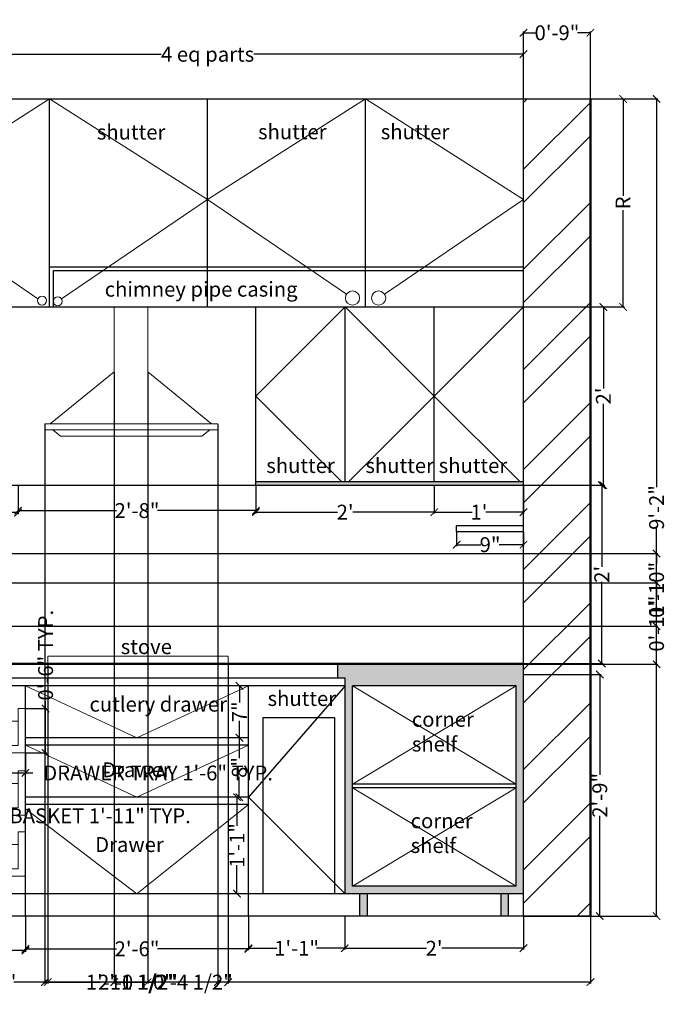
# Model space of a CAD drawing. Units: inches. Extents: x 3107 to 3291, y 1339 to 1621.
# Tile 3 of 3: x 3204 to 3291, y 1489 to 1621. Entities that reach past the tile are written whole.
import ezdxf

# ---------------------------------------------------------------- set-up
doc = ezdxf.new("R2010")
doc.units = ezdxf.units.IN
for name, color, linetype, lineweight in [('A-ANNO-DIMS', 2, 'Continuous', 18), ('A-ANNO-TEXT', 7, 'Continuous', 18), ('A-ELEV', 7, 'Continuous', 25), ('A-ELEV-OPEN', 165, 'Continuous', 13), ('A-ELEV-PATT', 8, 'Continuous', 13), ('A-EQPM', 3, 'Continuous', 18), ('A-FURN', 5, 'Continuous', 18), ('A-WALL', 7, 'Continuous', 50), ('A-WALL-PATT', 8, 'Continuous', 13)]:
    doc.layers.add(name, color=color, linetype=linetype, lineweight=lineweight)
doc.styles.get("Standard").update_dxf_attribs({"font": 'arial.ttf', "height": 2})
doc.dimstyles.get("Standard").update_dxf_attribs({"dimtxt": 2, "dimasz": 1, "dimexe": 0.18, "dimexo": 0.0625, "dimgap": 0.09, "dimtad": 0, "dimdec": 0, "dimzin": 0, "dimdsep": 46, "dimlunit": 3, "dimtxsty": 'Standard', "dimblk": 'ARCHTICK', "dimcen": 0.09, "dimadec": 0, "dimazin": 0, "dimtfac": 1, "dimtdec": 0, "dimtofl": 0, "dimtmove": 0, "dimatfit": 3, "dimfxl": 1, "dimtolj": 1, "dimtzin": 0, "dimarcsym": 0})

# ---------------------------------------------------------------- blocks, each defined once
blk = doc.blocks.new('_ArchTick')
at = {"color": 0, "linetype": 'ByBlock', "const_width": 0.15}
blk.add_lwpolyline([(-0.5, -0.5), (0.5, 0.5)], dxfattribs=at)
blk = doc.blocks.new('*D20')
at = {"layer": 'A-ANNO-DIMS', "color": 0, "lineweight": -2, "transparency": 16777216}
for p, q in [((3259.52, 1558.6), (3259.52, 1554.85)), ((3271.52, 1558.6), (3271.52, 1554.85)), ((3259.52, 1555.03), (3264.6, 1555.03)), ((3271.52, 1555.03), (3266.43, 1555.03))]:
    blk.add_line(p, q, dxfattribs=at)
at = {"layer": 'Defpoints', "color": 0, "transparency": 16777216}
for p in [(3259.52, 1558.66), (3271.52, 1558.66), (3259.52, 1555.03)]:
    blk.add_point(p, dxfattribs=at)
at = {"layer": 'A-ANNO-DIMS', "color": 0, "lineweight": -2, "transparency": 16777216, "rotation": 180}
blk.add_blockref('_ArchTick', (3259.52, 1555.03), dxfattribs=at)
at = {"layer": 'A-ANNO-DIMS', "color": 0, "lineweight": -2, "transparency": 16777216}
blk.add_blockref('_ArchTick', (3271.52, 1555.03), dxfattribs=at)
at = {"layer": 'A-ANNO-DIMS', "color": 0, "transparency": 16777216, "insert": (3265.52, 1555.03), "char_height": 2, "attachment_point": 5}
blk.add_mtext("\\A1;1'", dxfattribs=at)
blk = doc.blocks.new('*D21')
at = {"layer": 'A-ANNO-DIMS', "color": 0, "lineweight": -2, "transparency": 16777216}
for p, q in [((3235.52, 1558.6), (3235.52, 1554.85)), ((3259.52, 1558.6), (3259.52, 1554.85)), ((3235.52, 1555.03), (3246.49, 1555.03)), ((3259.52, 1555.03), (3248.54, 1555.03))]:
    blk.add_line(p, q, dxfattribs=at)
at = {"layer": 'Defpoints', "color": 0, "transparency": 16777216}
for p in [(3235.52, 1558.66), (3259.52, 1558.66), (3235.52, 1555.03)]:
    blk.add_point(p, dxfattribs=at)
at = {"layer": 'A-ANNO-DIMS', "color": 0, "lineweight": -2, "transparency": 16777216, "rotation": 180}
blk.add_blockref('_ArchTick', (3235.52, 1555.03), dxfattribs=at)
at = {"layer": 'A-ANNO-DIMS', "color": 0, "lineweight": -2, "transparency": 16777216}
blk.add_blockref('_ArchTick', (3259.52, 1555.03), dxfattribs=at)
at = {"layer": 'A-ANNO-DIMS', "color": 0, "transparency": 16777216, "insert": (3247.52, 1555.03), "char_height": 2, "attachment_point": 5}
blk.add_mtext("\\A1;2'", dxfattribs=at)
blk = doc.blocks.new('*D22')
at = {"layer": 'A-ANNO-DIMS', "color": 0, "lineweight": -2, "transparency": 16777216}
for p, q in [((3203.52, 1558.6), (3203.52, 1555.06)), ((3235.52, 1558.6), (3235.52, 1555.06)), ((3203.52, 1555.24), (3216.75, 1555.24)), ((3235.52, 1555.24), (3222.28, 1555.24))]:
    blk.add_line(p, q, dxfattribs=at)
at = {"layer": 'Defpoints', "color": 0, "transparency": 16777216}
for p in [(3203.52, 1558.66), (3235.52, 1558.66), (3203.52, 1555.24)]:
    blk.add_point(p, dxfattribs=at)
at = {"layer": 'A-ANNO-DIMS', "color": 0, "lineweight": -2, "transparency": 16777216, "rotation": 180}
blk.add_blockref('_ArchTick', (3203.52, 1555.24), dxfattribs=at)
at = {"layer": 'A-ANNO-DIMS', "color": 0, "lineweight": -2, "transparency": 16777216}
blk.add_blockref('_ArchTick', (3235.52, 1555.24), dxfattribs=at)
at = {"layer": 'A-ANNO-DIMS', "color": 0, "transparency": 16777216, "insert": (3219.52, 1555.24), "char_height": 2, "attachment_point": 5}
blk.add_mtext('\\A1;2\'-8"', dxfattribs=at)
blk = doc.blocks.new('*D23')
at = {"layer": 'A-ANNO-DIMS', "color": 0, "lineweight": -2, "transparency": 16777216}
for p, q in [((3186.52, 1558.6), (3186.52, 1554.78)), ((3203.52, 1558.6), (3203.52, 1554.78)), ((3186.52, 1554.96), (3192.36, 1554.96)), ((3203.52, 1554.96), (3197.67, 1554.96))]:
    blk.add_line(p, q, dxfattribs=at)
at = {"layer": 'Defpoints', "color": 0, "transparency": 16777216}
for p in [(3186.52, 1558.66), (3203.52, 1558.66), (3186.52, 1554.96)]:
    blk.add_point(p, dxfattribs=at)
at = {"layer": 'A-ANNO-DIMS', "color": 0, "lineweight": -2, "transparency": 16777216, "rotation": 180}
blk.add_blockref('_ArchTick', (3186.52, 1554.96), dxfattribs=at)
at = {"layer": 'A-ANNO-DIMS', "color": 0, "lineweight": -2, "transparency": 16777216}
blk.add_blockref('_ArchTick', (3203.52, 1554.96), dxfattribs=at)
at = {"layer": 'A-ANNO-DIMS', "color": 0, "transparency": 16777216, "insert": (3195.02, 1554.96), "char_height": 2, "attachment_point": 5}
blk.add_mtext('\\A1;1\'-5"', dxfattribs=at)
blk = doc.blocks.new('*D24')
at = {"layer": 'A-ANNO-DIMS', "color": 0, "lineweight": -2, "transparency": 16777216}
for p, q in [((3247.47, 1500.6), (3247.47, 1496.14)), ((3271.52, 1500.6), (3271.52, 1496.14)), ((3247.47, 1496.32), (3258.47, 1496.32)), ((3271.52, 1496.32), (3260.52, 1496.32))]:
    blk.add_line(p, q, dxfattribs=at)
at = {"layer": 'Defpoints', "color": 0, "transparency": 16777216}
for p in [(3247.47, 1500.66), (3271.52, 1500.66), (3247.47, 1496.32)]:
    blk.add_point(p, dxfattribs=at)
at = {"layer": 'A-ANNO-DIMS', "color": 0, "lineweight": -2, "transparency": 16777216, "rotation": 180}
blk.add_blockref('_ArchTick', (3247.47, 1496.32), dxfattribs=at)
at = {"layer": 'A-ANNO-DIMS', "color": 0, "lineweight": -2, "transparency": 16777216}
blk.add_blockref('_ArchTick', (3271.52, 1496.32), dxfattribs=at)
at = {"layer": 'A-ANNO-DIMS', "color": 0, "transparency": 16777216, "insert": (3259.49, 1496.32), "char_height": 2, "attachment_point": 5}
blk.add_mtext("\\A1;2'", dxfattribs=at)
blk = doc.blocks.new('*D25')
at = {"layer": 'A-ANNO-DIMS', "color": 0, "lineweight": -2, "transparency": 16777216}
for p, q in [((3234.52, 1500.6), (3234.52, 1496.14)), ((3247.47, 1500.6), (3247.47, 1496.14)), ((3234.52, 1496.32), (3238.34, 1496.32)), ((3247.47, 1496.32), (3243.65, 1496.32))]:
    blk.add_line(p, q, dxfattribs=at)
at = {"layer": 'Defpoints', "color": 0, "transparency": 16777216}
for p in [(3234.52, 1500.66), (3247.47, 1500.66), (3234.52, 1496.32)]:
    blk.add_point(p, dxfattribs=at)
at = {"layer": 'A-ANNO-DIMS', "color": 0, "lineweight": -2, "transparency": 16777216, "rotation": 180}
blk.add_blockref('_ArchTick', (3234.52, 1496.32), dxfattribs=at)
at = {"layer": 'A-ANNO-DIMS', "color": 0, "lineweight": -2, "transparency": 16777216}
blk.add_blockref('_ArchTick', (3247.47, 1496.32), dxfattribs=at)
at = {"layer": 'A-ANNO-DIMS', "color": 0, "transparency": 16777216, "insert": (3240.99, 1496.32), "char_height": 2, "attachment_point": 5}
blk.add_mtext('\\A1;1\'-1"', dxfattribs=at)
blk = doc.blocks.new('*D26')
at = {"layer": 'A-ANNO-DIMS', "color": 0, "lineweight": -2, "transparency": 16777216}
for p, q in [((3204.52, 1500.6), (3204.52, 1496.07)), ((3234.52, 1500.6), (3234.52, 1496.07)), ((3204.52, 1496.25), (3216.75, 1496.25)), ((3234.52, 1496.25), (3222.28, 1496.25))]:
    blk.add_line(p, q, dxfattribs=at)
at = {"layer": 'Defpoints', "color": 0, "transparency": 16777216}
for p in [(3204.52, 1500.66), (3234.52, 1500.66), (3204.52, 1496.25)]:
    blk.add_point(p, dxfattribs=at)
at = {"layer": 'A-ANNO-DIMS', "color": 0, "lineweight": -2, "transparency": 16777216, "rotation": 180}
blk.add_blockref('_ArchTick', (3204.52, 1496.25), dxfattribs=at)
at = {"layer": 'A-ANNO-DIMS', "color": 0, "lineweight": -2, "transparency": 16777216}
blk.add_blockref('_ArchTick', (3234.52, 1496.25), dxfattribs=at)
at = {"layer": 'A-ANNO-DIMS', "color": 0, "transparency": 16777216, "insert": (3219.52, 1496.25), "char_height": 2, "attachment_point": 5}
blk.add_mtext('\\A1;2\'-6"', dxfattribs=at)
blk = doc.blocks.new('*D27')
at = {"layer": 'A-ANNO-DIMS', "color": 0, "lineweight": -2, "transparency": 16777216}
for p, q in [((3186.52, 1500.6), (3186.52, 1495.83)), ((3204.52, 1500.6), (3204.52, 1495.83)), ((3186.52, 1496.01), (3192.86, 1496.01)), ((3204.52, 1496.01), (3198.17, 1496.01))]:
    blk.add_line(p, q, dxfattribs=at)
at = {"layer": 'Defpoints', "color": 0, "transparency": 16777216}
for p in [(3186.52, 1500.66), (3204.52, 1500.66), (3186.52, 1496.01)]:
    blk.add_point(p, dxfattribs=at)
at = {"layer": 'A-ANNO-DIMS', "color": 0, "lineweight": -2, "transparency": 16777216, "rotation": 180}
blk.add_blockref('_ArchTick', (3186.52, 1496.01), dxfattribs=at)
at = {"layer": 'A-ANNO-DIMS', "color": 0, "lineweight": -2, "transparency": 16777216}
blk.add_blockref('_ArchTick', (3204.52, 1496.01), dxfattribs=at)
at = {"layer": 'A-ANNO-DIMS', "color": 0, "transparency": 16777216, "insert": (3195.52, 1496.01), "char_height": 2, "attachment_point": 5}
blk.add_mtext('\\A1;1\'-6"', dxfattribs=at)
blk = doc.blocks.new('*D30')
at = {"layer": 'A-ANNO-DIMS', "color": 0, "lineweight": -2, "transparency": 16777216}
for p, q in [((3271.58, 1533.17), (3281.96, 1533.17)), ((3281.78, 1533.17), (3281.78, 1519.68)), ((3281.78, 1500.66), (3281.78, 1514.15)), ((3271.58, 1500.66), (3281.96, 1500.66))]:
    blk.add_line(p, q, dxfattribs=at)
at = {"layer": 'Defpoints', "color": 0, "transparency": 16777216}
for p in [(3271.52, 1533.17), (3281.78, 1533.17), (3271.52, 1500.66)]:
    blk.add_point(p, dxfattribs=at)
at = {"layer": 'A-ANNO-DIMS', "color": 0, "lineweight": -2, "transparency": 16777216}
for p, rotation in [((3281.78, 1533.17), 90), ((3281.78, 1500.66), 270)]:
    blk.add_blockref('_ArchTick', p, dxfattribs=dict(at, rotation=rotation))
at = {"layer": 'A-ANNO-DIMS', "color": 0, "transparency": 16777216, "insert": (3281.78, 1516.91), "char_height": 2, "attachment_point": 5, "rotation": 90}
blk.add_mtext('\\A1;2\'-9"', dxfattribs=at)
blk = doc.blocks.new('*D31')
at = {"layer": 'A-ANNO-DIMS', "color": 0, "lineweight": -2, "transparency": 16777216}
for p, q in [((3271.58, 1558.66), (3282.23, 1558.66)), ((3282.05, 1558.66), (3282.05, 1547.69)), ((3282.05, 1534.66), (3282.05, 1545.63)), ((3271.58, 1534.66), (3282.23, 1534.66))]:
    blk.add_line(p, q, dxfattribs=at)
at = {"layer": 'Defpoints', "color": 0, "transparency": 16777216}
for p in [(3271.52, 1558.66), (3282.05, 1558.66), (3271.52, 1534.66)]:
    blk.add_point(p, dxfattribs=at)
at = {"layer": 'A-ANNO-DIMS', "color": 0, "lineweight": -2, "transparency": 16777216}
for p, rotation in [((3282.05, 1558.66), 90), ((3282.05, 1534.66), 270)]:
    blk.add_blockref('_ArchTick', p, dxfattribs=dict(at, rotation=rotation))
at = {"layer": 'A-ANNO-DIMS', "color": 0, "transparency": 16777216, "insert": (3282.05, 1546.66), "char_height": 2, "attachment_point": 5, "rotation": 90}
blk.add_mtext("\\A1;2'", dxfattribs=at)
blk = doc.blocks.new('*D32')
at = {"layer": 'A-ANNO-DIMS', "color": 0, "lineweight": -2, "transparency": 16777216}
for p, q in [((3271.58, 1582.66), (3282.44, 1582.66)), ((3282.26, 1582.66), (3282.26, 1571.69)), ((3282.26, 1558.66), (3282.26, 1569.63)), ((3271.58, 1558.66), (3282.44, 1558.66))]:
    blk.add_line(p, q, dxfattribs=at)
at = {"layer": 'Defpoints', "color": 0, "transparency": 16777216}
for p in [(3271.52, 1582.66), (3282.26, 1582.66), (3271.52, 1558.66)]:
    blk.add_point(p, dxfattribs=at)
at = {"layer": 'A-ANNO-DIMS', "color": 0, "lineweight": -2, "transparency": 16777216}
for p, rotation in [((3282.26, 1582.66), 90), ((3282.26, 1558.66), 270)]:
    blk.add_blockref('_ArchTick', p, dxfattribs=dict(at, rotation=rotation))
at = {"layer": 'A-ANNO-DIMS', "color": 0, "transparency": 16777216, "insert": (3282.26, 1570.66), "char_height": 2, "attachment_point": 5, "rotation": 90}
blk.add_mtext("\\A1;2'", dxfattribs=at)
blk = doc.blocks.new('*D33')
at = {"layer": 'A-ANNO-DIMS', "color": 0, "lineweight": -2, "transparency": 16777216}
for p, q in [((3271.58, 1610.66), (3285.09, 1610.66)), ((3284.91, 1610.66), (3284.91, 1597.63)), ((3284.91, 1582.66), (3284.91, 1595.69)), ((3271.58, 1582.66), (3285.09, 1582.66))]:
    blk.add_line(p, q, dxfattribs=at)
at = {"layer": 'Defpoints', "color": 0, "transparency": 16777216}
for p in [(3271.52, 1610.66), (3284.91, 1610.66), (3271.52, 1582.66)]:
    blk.add_point(p, dxfattribs=at)
at = {"layer": 'A-ANNO-DIMS', "color": 0, "lineweight": -2, "transparency": 16777216}
for p, rotation in [((3284.91, 1610.66), 90), ((3284.91, 1582.66), 270)]:
    blk.add_blockref('_ArchTick', p, dxfattribs=dict(at, rotation=rotation))
at = {"layer": 'A-ANNO-DIMS', "color": 0, "transparency": 16777216, "insert": (3284.91, 1596.66), "char_height": 2, "attachment_point": 5, "rotation": 90}
blk.add_mtext('\\A1;R ', dxfattribs=at)
blk = doc.blocks.new('*D34')
at = {"layer": 'A-ANNO-DIMS', "color": 0, "lineweight": -2, "transparency": 16777216}
for p, q in [((3186.52, 1610.72), (3186.52, 1616.85)), ((3186.52, 1616.67), (3222.79, 1616.67)), ((3271.52, 1616.67), (3235.25, 1616.67)), ((3271.52, 1610.72), (3271.52, 1616.85))]:
    blk.add_line(p, q, dxfattribs=at)
at = {"layer": 'Defpoints', "color": 0, "transparency": 16777216}
for p in [(3186.52, 1616.67), (3186.52, 1610.66), (3271.52, 1610.66)]:
    blk.add_point(p, dxfattribs=at)
at = {"layer": 'A-ANNO-DIMS', "color": 0, "lineweight": -2, "transparency": 16777216, "rotation": 180}
blk.add_blockref('_ArchTick', (3186.52, 1616.67), dxfattribs=at)
at = {"layer": 'A-ANNO-DIMS', "color": 0, "lineweight": -2, "transparency": 16777216}
blk.add_blockref('_ArchTick', (3271.52, 1616.67), dxfattribs=at)
at = {"layer": 'A-ANNO-DIMS', "color": 0, "transparency": 16777216, "insert": (3229.02, 1616.67), "char_height": 2, "attachment_point": 5}
blk.add_mtext('\\A1;4 eq parts', dxfattribs=at)
blk = doc.blocks.new('*D39')
at = {"layer": 'A-ANNO-DIMS', "color": 0, "lineweight": -2, "transparency": 16777216}
for p, q in [((3262.52, 1552.37), (3262.52, 1550.47)), ((3271.52, 1552.37), (3271.52, 1550.47)), ((3262.52, 1550.65), (3265.78, 1550.65)), ((3271.52, 1550.65), (3268.26, 1550.65))]:
    blk.add_line(p, q, dxfattribs=at)
at = {"layer": 'Defpoints', "color": 0, "transparency": 16777216}
for p in [(3262.52, 1552.43), (3271.52, 1552.43), (3262.52, 1550.65)]:
    blk.add_point(p, dxfattribs=at)
at = {"layer": 'A-ANNO-DIMS', "color": 0, "lineweight": -2, "transparency": 16777216, "rotation": 180}
blk.add_blockref('_ArchTick', (3262.52, 1550.65), dxfattribs=at)
at = {"layer": 'A-ANNO-DIMS', "color": 0, "lineweight": -2, "transparency": 16777216}
blk.add_blockref('_ArchTick', (3271.52, 1550.65), dxfattribs=at)
at = {"layer": 'A-ANNO-DIMS', "color": 0, "transparency": 16777216, "insert": (3267.02, 1550.65), "char_height": 2, "attachment_point": 5}
blk.add_mtext('\\A1;9"', dxfattribs=at)
blk = doc.blocks.new('*D45')
at = {"layer": 'A-ANNO-DIMS', "color": 0, "lineweight": -2, "transparency": 16777216}
for p, q in [((3234.46, 1531.66), (3233.13, 1531.66)), ((3233.31, 1531.66), (3233.31, 1529.39)), ((3233.31, 1524.66), (3233.31, 1526.93)), ((3234.46, 1524.66), (3233.13, 1524.66))]:
    blk.add_line(p, q, dxfattribs=at)
at = {"layer": 'Defpoints', "color": 0, "transparency": 16777216}
for p in [(3233.31, 1531.66), (3234.52, 1531.66), (3234.52, 1524.66)]:
    blk.add_point(p, dxfattribs=at)
at = {"layer": 'A-ANNO-DIMS', "color": 0, "lineweight": -2, "transparency": 16777216}
for p, rotation in [((3233.31, 1531.66), 90), ((3233.31, 1524.66), 270)]:
    blk.add_blockref('_ArchTick', p, dxfattribs=dict(at, rotation=rotation))
at = {"layer": 'A-ANNO-DIMS', "color": 0, "transparency": 16777216, "insert": (3233.31, 1528.16), "char_height": 2, "attachment_point": 5, "rotation": 90}
blk.add_mtext('\\A1;7"', dxfattribs=at)
blk = doc.blocks.new('*D46')
at = {"layer": 'A-ANNO-DIMS', "color": 0, "lineweight": -2, "transparency": 16777216}
for p, q in [((3234.46, 1524.66), (3233.1, 1524.66)), ((3233.28, 1524.66), (3233.28, 1521.9)), ((3233.28, 1516.66), (3233.28, 1519.42)), ((3234.46, 1516.66), (3233.1, 1516.66))]:
    blk.add_line(p, q, dxfattribs=at)
at = {"layer": 'Defpoints', "color": 0, "transparency": 16777216}
for p in [(3234.52, 1524.66), (3233.28, 1516.66), (3234.52, 1516.66)]:
    blk.add_point(p, dxfattribs=at)
at = {"layer": 'A-ANNO-DIMS', "color": 0, "lineweight": -2, "transparency": 16777216}
for p, rotation in [((3233.28, 1524.66), 90), ((3233.28, 1516.66), 270)]:
    blk.add_blockref('_ArchTick', p, dxfattribs=dict(at, rotation=rotation))
at = {"layer": 'A-ANNO-DIMS', "color": 0, "transparency": 16777216, "insert": (3233.28, 1520.66), "char_height": 2, "attachment_point": 5, "rotation": 90}
blk.add_mtext('\\A1;8"', dxfattribs=at)
blk = doc.blocks.new('*D47')
at = {"layer": 'A-ANNO-DIMS', "color": 0, "lineweight": -2, "transparency": 16777216}
for p, q in [((3234.46, 1516.66), (3232.79, 1516.66)), ((3232.97, 1516.66), (3232.97, 1512.81)), ((3232.97, 1503.66), (3232.97, 1507.5)), ((3234.46, 1503.66), (3232.79, 1503.66))]:
    blk.add_line(p, q, dxfattribs=at)
at = {"layer": 'Defpoints', "color": 0, "transparency": 16777216}
for p in [(3234.52, 1516.66), (3232.97, 1503.66), (3234.52, 1503.66)]:
    blk.add_point(p, dxfattribs=at)
at = {"layer": 'A-ANNO-DIMS', "color": 0, "lineweight": -2, "transparency": 16777216}
for p, rotation in [((3232.97, 1516.66), 90), ((3232.97, 1503.66), 270)]:
    blk.add_blockref('_ArchTick', p, dxfattribs=dict(at, rotation=rotation))
at = {"layer": 'A-ANNO-DIMS', "color": 0, "transparency": 16777216, "insert": (3232.97, 1510.16), "char_height": 2, "attachment_point": 5, "rotation": 90}
blk.add_mtext('\\A1;1\'-1"', dxfattribs=at)
blk = doc.blocks.new('DRAWER-TRAY')
for p, q in [((3186.52, 1528.59), (3187.52, 1528.59)), ((3186.52, 1522.62), (3186.52, 1528.59)), ((3187.52, 1523.62), (3187.52, 1528.59)), ((3203.52, 1528.59), (3203.52, 1523.62)), ((3203.52, 1528.59), (3204.52, 1528.59)), ((3204.52, 1528.59), (3204.52, 1522.62)), ((3187.52, 1526.9), (3203.52, 1526.9)), ((3203.52, 1523.62), (3187.52, 1523.62)), ((3204.52, 1522.62), (3186.52, 1522.62))]:
    blk.add_line(p, q)
blk = doc.blocks.new('*D50')
at = {"layer": 'A-ANNO-DIMS', "color": 0, "lineweight": -2, "transparency": 16777216}
for p, q in [((3186.52, 1522.56), (3186.52, 1519.74)), ((3204.52, 1522.56), (3204.52, 1519.74)), ((3186.52, 1519.92), (3204.52, 1519.92)), ((3204.52, 1519.92), (3205.52, 1519.92))]:
    blk.add_line(p, q, dxfattribs=at)
at = {"layer": 'Defpoints', "color": 0, "transparency": 16777216}
for p in [(3186.52, 1522.62), (3204.52, 1522.62), (3204.52, 1519.92)]:
    blk.add_point(p, dxfattribs=at)
at = {"layer": 'A-ANNO-DIMS', "color": 0, "lineweight": -2, "transparency": 16777216, "rotation": 180}
blk.add_blockref('_ArchTick', (3186.52, 1519.92), dxfattribs=at)
at = {"layer": 'A-ANNO-DIMS', "color": 0, "lineweight": -2, "transparency": 16777216}
blk.add_blockref('_ArchTick', (3204.52, 1519.92), dxfattribs=at)
at = {"layer": 'A-ANNO-DIMS', "color": 0, "transparency": 16777216, "insert": (3222.36, 1519.92), "char_height": 2, "attachment_point": 5}
blk.add_mtext('\\A1;DRAWER TRAY 1\'-6" TYP.', dxfattribs=at)
blk = doc.blocks.new('*D51')
at = {"layer": 'A-ANNO-DIMS', "color": 0, "lineweight": -2, "transparency": 16777216}
for p, q in [((3204.58, 1528.59), (3207.4, 1528.59)), ((3207.22, 1528.59), (3207.22, 1529.59)), ((3207.22, 1522.62), (3207.22, 1528.59)), ((3204.58, 1522.62), (3207.4, 1522.62))]:
    blk.add_line(p, q, dxfattribs=at)
at = {"layer": 'Defpoints', "color": 0, "transparency": 16777216}
for p in [(3204.52, 1528.59), (3207.22, 1528.59), (3204.52, 1522.62)]:
    blk.add_point(p, dxfattribs=at)
at = {"layer": 'A-ANNO-DIMS', "color": 0, "lineweight": -2, "transparency": 16777216}
for p, rotation in [((3207.22, 1528.59), 90), ((3207.22, 1522.62), 270)]:
    blk.add_blockref('_ArchTick', p, dxfattribs=dict(at, rotation=rotation))
at = {"layer": 'A-ANNO-DIMS', "color": 0, "transparency": 16777216, "insert": (3207.22, 1535.77), "char_height": 2, "attachment_point": 5, "rotation": 90}
blk.add_mtext('\\A1;0\'-6" TYP.', dxfattribs=at)
blk = doc.blocks.new('*D52')
at = {"layer": 'A-ANNO-DIMS', "color": 0, "lineweight": -2, "transparency": 16777216}
for p, q in [((3163.52, 1517.53), (3163.52, 1513.97)), ((3186.52, 1517.53), (3186.52, 1513.97)), ((3163.52, 1514.15), (3186.52, 1514.15)), ((3186.52, 1514.15), (3187.52, 1514.15))]:
    blk.add_line(p, q, dxfattribs=at)
at = {"layer": 'Defpoints', "color": 0, "transparency": 16777216}
for p in [(3163.52, 1517.6), (3186.52, 1517.6), (3186.52, 1514.15)]:
    blk.add_point(p, dxfattribs=at)
at = {"layer": 'A-ANNO-DIMS', "color": 0, "lineweight": -2, "transparency": 16777216, "rotation": 180}
blk.add_blockref('_ArchTick', (3163.52, 1514.15), dxfattribs=at)
at = {"layer": 'A-ANNO-DIMS', "color": 0, "lineweight": -2, "transparency": 16777216}
blk.add_blockref('_ArchTick', (3186.52, 1514.15), dxfattribs=at)
at = {"layer": 'A-ANNO-DIMS', "color": 0, "transparency": 16777216, "insert": (3207.63, 1514.15), "char_height": 2, "attachment_point": 5}
blk.add_mtext('\\A1;PULL-OUT BASKET 1\'-11" TYP.', dxfattribs=at)
blk = doc.blocks.new('*D56')
at = {"layer": 'A-ANNO-DIMS', "color": 0, "lineweight": -2, "transparency": 16777216}
for p, q in [((3280.58, 1610.66), (3289.6, 1610.66)), ((3289.42, 1610.66), (3289.42, 1558.41)), ((3289.42, 1500.66), (3289.42, 1552.91)), ((3280.58, 1500.66), (3289.6, 1500.66))]:
    blk.add_line(p, q, dxfattribs=at)
at = {"layer": 'Defpoints', "color": 0, "transparency": 16777216}
for p in [(3280.52, 1610.66), (3289.42, 1610.66), (3280.52, 1500.66)]:
    blk.add_point(p, dxfattribs=at)
at = {"layer": 'A-ANNO-DIMS', "color": 0, "lineweight": -2, "transparency": 16777216}
for p, rotation in [((3289.42, 1610.66), 90), ((3289.42, 1500.66), 270)]:
    blk.add_blockref('_ArchTick', p, dxfattribs=dict(at, rotation=rotation))
at = {"layer": 'A-ANNO-DIMS', "color": 0, "transparency": 16777216, "insert": (3289.42, 1555.66), "char_height": 2, "attachment_point": 5, "rotation": 90}
blk.add_mtext('\\A1;9\'-2"', dxfattribs=at)
blk = doc.blocks.new('*D59')
at = {"layer": 'A-ANNO-DIMS', "color": 0, "lineweight": -2, "transparency": 16777216}
for p, q in [((3271.52, 1610.72), (3271.52, 1619.74)), ((3280.52, 1610.72), (3280.52, 1619.74)), ((3271.52, 1619.56), (3273.27, 1619.56)), ((3280.52, 1619.56), (3278.77, 1619.56))]:
    blk.add_line(p, q, dxfattribs=at)
at = {"layer": 'Defpoints', "color": 0, "transparency": 16777216}
for p in [(3280.52, 1619.56), (3271.52, 1610.66), (3280.52, 1610.66)]:
    blk.add_point(p, dxfattribs=at)
at = {"layer": 'A-ANNO-DIMS', "color": 0, "lineweight": -2, "transparency": 16777216, "rotation": 180}
blk.add_blockref('_ArchTick', (3271.52, 1619.56), dxfattribs=at)
at = {"layer": 'A-ANNO-DIMS', "color": 0, "lineweight": -2, "transparency": 16777216}
blk.add_blockref('_ArchTick', (3280.52, 1619.56), dxfattribs=at)
at = {"layer": 'A-ANNO-DIMS', "color": 0, "transparency": 16777216, "insert": (3276.02, 1619.56), "char_height": 2, "attachment_point": 5}
blk.add_mtext('\\A1;0\'-9"', dxfattribs=at)
blk = doc.blocks.new('*D62')
at = {"layer": 'A-ANNO-DIMS', "color": 0, "lineweight": -2, "transparency": 16777216}
for p, q in [((3140.37, 1549.46), (3289.6, 1549.46)), ((3289.42, 1549.46), (3289.42, 1548.09)), ((3289.42, 1539.66), (3289.42, 1541.04)), ((3140.87, 1539.66), (3289.6, 1539.66))]:
    blk.add_line(p, q, dxfattribs=at)
at = {"layer": 'Defpoints', "color": 0, "transparency": 16777216}
for p in [(3140.3, 1549.46), (3289.42, 1549.46), (3140.8, 1539.66)]:
    blk.add_point(p, dxfattribs=at)
at = {"layer": 'A-ANNO-DIMS', "color": 0, "lineweight": -2, "transparency": 16777216}
for p, rotation in [((3289.42, 1549.46), 90), ((3289.42, 1539.66), 270)]:
    blk.add_blockref('_ArchTick', p, dxfattribs=dict(at, rotation=rotation))
at = {"layer": 'A-ANNO-DIMS', "color": 0, "transparency": 16777216, "insert": (3289.42, 1544.56), "char_height": 2, "attachment_point": 5, "rotation": 90}
blk.add_mtext('\\A1;0\'-10"', dxfattribs=at)
blk = doc.blocks.new('*D63')
at = {"layer": 'A-ANNO-DIMS', "color": 0, "lineweight": -2, "transparency": 16777216}
for p, q in [((3184.88, 1545.5), (3289.6, 1545.5)), ((3289.42, 1545.5), (3289.42, 1543.55)), ((3289.42, 1534.55), (3289.42, 1536.5)), ((3184.88, 1534.55), (3289.6, 1534.55))]:
    blk.add_line(p, q, dxfattribs=at)
at = {"layer": 'Defpoints', "color": 0, "transparency": 16777216}
for p in [(3184.82, 1545.5), (3289.42, 1545.5), (3184.82, 1534.55)]:
    blk.add_point(p, dxfattribs=at)
at = {"layer": 'A-ANNO-DIMS', "color": 0, "lineweight": -2, "transparency": 16777216}
for p, rotation in [((3289.42, 1545.5), 90), ((3289.42, 1534.55), 270)]:
    blk.add_blockref('_ArchTick', p, dxfattribs=dict(at, rotation=rotation))
at = {"layer": 'A-ANNO-DIMS', "color": 0, "transparency": 16777216, "insert": (3289.42, 1540.02), "char_height": 2, "attachment_point": 5, "rotation": 90}
blk.add_mtext('\\A1;0\'-11"', dxfattribs=at)
blk = doc.blocks.new('*D64')
at = {"layer": 'A-ANNO-DIMS', "color": 0, "lineweight": -2, "transparency": 16777216}
for p, q in [((3207.13, 1566.85), (3207.13, 1491.58)), ((3230.39, 1566.85), (3230.39, 1491.58)), ((3207.13, 1491.76), (3213, 1491.76)), ((3230.39, 1491.76), (3224.52, 1491.76))]:
    blk.add_line(p, q, dxfattribs=at)
at = {"layer": 'Defpoints', "color": 0, "transparency": 16777216}
for p in [(3207.13, 1566.91), (3230.39, 1566.91), (3230.39, 1491.76)]:
    blk.add_point(p, dxfattribs=at)
at = {"layer": 'A-ANNO-DIMS', "color": 0, "lineweight": -2, "transparency": 16777216, "rotation": 180}
blk.add_blockref('_ArchTick', (3207.13, 1491.76), dxfattribs=at)
at = {"layer": 'A-ANNO-DIMS', "color": 0, "lineweight": -2, "transparency": 16777216}
blk.add_blockref('_ArchTick', (3230.39, 1491.76), dxfattribs=at)
at = {"layer": 'A-ANNO-DIMS', "color": 0, "transparency": 16777216, "insert": (3218.76, 1491.76), "char_height": 2, "attachment_point": 5}
blk.add_mtext('\\A1;1\'-11 1/2"', dxfattribs=at)
blk = doc.blocks.new('*D65')
at = {"layer": 'A-ANNO-DIMS', "color": 0, "lineweight": -2, "transparency": 16777216}
for p, q in [((3216.45, 1573.85), (3216.45, 1491.58)), ((3220.96, 1573.85), (3220.96, 1491.58)), ((3216.45, 1491.76), (3220.96, 1491.76)), ((3220.96, 1491.76), (3221.96, 1491.76))]:
    blk.add_line(p, q, dxfattribs=at)
at = {"layer": 'Defpoints', "color": 0, "transparency": 16777216}
for p in [(3216.45, 1573.91), (3220.96, 1573.91), (3220.96, 1491.76)]:
    blk.add_point(p, dxfattribs=at)
at = {"layer": 'A-ANNO-DIMS', "color": 0, "lineweight": -2, "transparency": 16777216, "rotation": 180}
blk.add_blockref('_ArchTick', (3216.45, 1491.76), dxfattribs=at)
at = {"layer": 'A-ANNO-DIMS', "color": 0, "lineweight": -2, "transparency": 16777216}
blk.add_blockref('_ArchTick', (3220.96, 1491.76), dxfattribs=at)
at = {"layer": 'A-ANNO-DIMS', "color": 0, "transparency": 16777216, "insert": (3227.04, 1491.76), "char_height": 2, "attachment_point": 5}
blk.add_mtext('\\A1;0\'-4 1/2"', dxfattribs=at)
blk = doc.blocks.new('*D66')
at = {"layer": 'A-ANNO-DIMS', "color": 0, "lineweight": -2, "transparency": 16777216}
for p, q in [((3207.51, 1534.6), (3207.51, 1491.58)), ((3231.79, 1534.6), (3231.79, 1491.58)), ((3207.51, 1491.76), (3214.55, 1491.76)), ((3231.79, 1491.76), (3224.75, 1491.76))]:
    blk.add_line(p, q, dxfattribs=at)
at = {"layer": 'Defpoints', "color": 0, "transparency": 16777216}
for p in [(3207.51, 1534.66), (3231.79, 1534.66), (3231.79, 1491.76)]:
    blk.add_point(p, dxfattribs=at)
at = {"layer": 'A-ANNO-DIMS', "color": 0, "lineweight": -2, "transparency": 16777216, "rotation": 180}
blk.add_blockref('_ArchTick', (3207.51, 1491.76), dxfattribs=at)
at = {"layer": 'A-ANNO-DIMS', "color": 0, "lineweight": -2, "transparency": 16777216}
blk.add_blockref('_ArchTick', (3231.79, 1491.76), dxfattribs=at)
at = {"layer": 'A-ANNO-DIMS', "color": 0, "transparency": 16777216, "insert": (3219.65, 1491.76), "char_height": 2, "attachment_point": 5}
blk.add_mtext('\\A1;2\'-0 1/2"', dxfattribs=at)
blk = doc.blocks.new('*D67')
at = {"layer": 'A-ANNO-DIMS', "color": 0, "lineweight": -2, "transparency": 16777216}
for p, q in [((3118.52, 1500.6), (3118.52, 1491.58)), ((3280.52, 1500.6), (3280.52, 1491.58)), ((3118.52, 1491.76), (3196.09, 1491.76)), ((3280.52, 1491.76), (3202.95, 1491.76))]:
    blk.add_line(p, q, dxfattribs=at)
at = {"layer": 'Defpoints', "color": 0, "transparency": 16777216}
for p in [(3118.52, 1500.66), (3280.52, 1500.66), (3280.52, 1491.76)]:
    blk.add_point(p, dxfattribs=at)
at = {"layer": 'A-ANNO-DIMS', "color": 0, "lineweight": -2, "transparency": 16777216, "rotation": 180}
blk.add_blockref('_ArchTick', (3118.52, 1491.76), dxfattribs=at)
at = {"layer": 'A-ANNO-DIMS', "color": 0, "lineweight": -2, "transparency": 16777216}
blk.add_blockref('_ArchTick', (3280.52, 1491.76), dxfattribs=at)
at = {"layer": 'A-ANNO-DIMS', "color": 0, "transparency": 16777216, "insert": (3199.52, 1491.76), "char_height": 2, "attachment_point": 5}
blk.add_mtext('\\A1;13\'-6"', dxfattribs=at)

msp = doc.modelspace()

# ---------------------------------------------------------------- hatches: boundary and pattern name
at = {"layer": 'A-ELEV-PATT'}
h = msp.add_hatch(color=256, dxfattribs=at)
h.dxf.hatch_style = 1
h.paths.add_polyline_path([(3271.52, 1559.16), (3235.52, 1559.16), (3235.52, 1558.66), (3271.52, 1558.66)])
h = msp.add_hatch(color=256, dxfattribs=at)
h.dxf.hatch_style = 1
h.paths.add_polyline_path([(3271.52, 1534.66), (3246.53, 1534.66), (3246.53, 1532.66), (3247.52, 1532.66), (3247.52, 1503.66), (3271.52, 1503.66)])
h.paths.add_polyline_path([(3270.52, 1504.66), (3248.52, 1504.66), (3248.52, 1531.66), (3270.52, 1531.66)], flags=16)
h.paths.add_polyline_path([(3259.52, 1525.03), (3270.52, 1518.41), (3248.52, 1518.41)], flags=0)
h.paths.add_polyline_path([(3270.52, 1517.91), (3259.52, 1511.28), (3248.52, 1517.91)], flags=0)
h = msp.add_hatch(color=256, dxfattribs=at)
h.dxf.hatch_style = 1
h.paths.add_polyline_path([(3269.52, 1503.66), (3268.52, 1503.66), (3268.52, 1500.66), (3269.52, 1500.66)])
h.paths.add_polyline_path([(3249.52, 1500.66), (3250.52, 1500.66), (3250.52, 1503.66), (3249.52, 1503.66)])
at = {"layer": 'A-WALL-PATT'}
h = msp.add_hatch(dxfattribs=at)
h.set_pattern_fill('ANSI32', color=256)
h.paths.add_polyline_path([(3280.52, 1582.66), (3280.52, 1610.66), (3271.52, 1610.66), (3271.52, 1534.66), (3271.52, 1500.66), (3280.52, 1500.66)])
h.paths.add_polyline_path([(3127.52, 1582.66), (3118.52, 1582.66), (3118.52, 1500.66), (3127.52, 1500.66)])
h.paths.add_polyline_path([(3127.52, 1610.66), (3118.52, 1610.66), (3118.52, 1582.66), (3127.52, 1582.66)])

# ---------------------------------------------------------------- linework, layer by layer
at = {"layer": 'A-ELEV'}
for p, q in [((3118.52, 1610.66), (3280.52, 1610.66)), ((3207.77, 1582.66), (3207.77, 1610.66)), ((3229.02, 1582.66), (3229.02, 1610.66)), ((3250.27, 1582.66), (3250.27, 1610.66)), ((3271.52, 1534.66), (3271.52, 1610.66)), ((3207.77, 1588.05), (3271.52, 1588.05)), ((3208.27, 1587.55), (3271.52, 1587.55)), ((3208.27, 1582.66), (3208.27, 1587.55)), ((3127.52, 1582.66), (3271.52, 1582.66)), ((3235.52, 1558.66), (3235.52, 1582.66)), ((3247.52, 1559.16), (3247.52, 1582.66)), ((3259.52, 1559.16), (3259.52, 1582.66)), ((3235.52, 1559.16), (3271.52, 1559.16)), ((3186.52, 1558.66), (3271.52, 1558.66)), ((3271.52, 1553.2), (3262.52, 1553.2)), ((3262.52, 1552.43), (3262.52, 1553.2)), ((3262.52, 1552.43), (3271.52, 1552.43)), ((3271.52, 1552.43), (3271.52, 1553.2)), ((3271.52, 1534.66), (3186.52, 1534.66)), ((3246.53, 1532.66), (3246.53, 1534.66)), ((3271.52, 1500.66), (3271.52, 1534.66)), ((3247.52, 1532.66), (3186.52, 1532.66)), ((3247.52, 1503.66), (3247.52, 1532.66)), ((3247.52, 1531.66), (3186.52, 1531.66)), ((3204.52, 1500.66), (3204.52, 1531.66)), ((3234.52, 1500.66), (3234.52, 1531.66)), ((3247.52, 1531.66), (3234.52, 1516.66)), ((3248.52, 1504.66), (3248.52, 1531.66)), ((3270.52, 1531.66), (3248.52, 1531.66)), ((3270.52, 1504.66), (3270.52, 1531.66)), ((3234.52, 1524.66), (3204.52, 1524.66)), ((3234.52, 1523.66), (3204.52, 1523.66)), ((3270.52, 1518.41), (3248.52, 1518.41)), ((3270.52, 1517.91), (3248.52, 1517.91)), ((3234.52, 1516.66), (3204.52, 1516.66)), ((3234.52, 1516.66), (3247.52, 1503.66)), ((3234.52, 1515.66), (3204.52, 1515.66)), ((3270.52, 1504.66), (3248.52, 1504.66)), ((3204.52, 1503.66), (3162.52, 1503.66)), ((3234.52, 1503.66), (3204.52, 1503.66)), ((3271.52, 1503.66), (3234.52, 1503.66)), ((3249.52, 1500.66), (3249.52, 1503.66)), ((3250.52, 1500.66), (3250.52, 1503.66)), ((3268.52, 1500.66), (3268.52, 1503.66)), ((3269.52, 1500.66), (3269.52, 1503.66)), ((3280.52, 1500.66), (3118.52, 1500.66))]:
    msp.add_line(p, q, dxfattribs=at)
msp.add_lwpolyline([(3236.48, 1527.4), (3246.1, 1527.4), (3246.1, 1503.66), (3236.48, 1503.66)], close=True, dxfattribs=at)
at = {"layer": 'A-ELEV-OPEN'}
for p, q in [((3207.77, 1610.66), (3186.52, 1597.16)), ((3229.02, 1597.12), (3207.77, 1610.66)), ((3229.02, 1597.12), (3250.27, 1610.66)), ((3271.52, 1597.12), (3250.27, 1610.66)), ((3186.52, 1597.16), (3206.19, 1583.74)), ((3209.36, 1583.74), (3229.02, 1597.12)), ((3247.72, 1584.39), (3229.02, 1597.12)), ((3252.81, 1584.39), (3271.52, 1597.12)), ((3247.52, 1582.66), (3235.52, 1570.66)), ((3247.52, 1582.66), (3259.52, 1570.66)), ((3271.52, 1582.66), (3259.52, 1570.66)), ((3235.52, 1570.66), (3247.02, 1559.16)), ((3259.52, 1570.66), (3248.02, 1559.16)), ((3259.52, 1570.66), (3271.02, 1559.16)), ((3204.52, 1531.66), (3219.52, 1524.66)), ((3219.52, 1524.66), (3234.52, 1531.66)), ((3270.52, 1518.41), (3248.52, 1531.66)), ((3270.52, 1531.66), (3248.52, 1518.41)), ((3204.52, 1523.66), (3219.52, 1516.66)), ((3219.52, 1516.66), (3234.52, 1523.66)), ((3270.52, 1504.66), (3248.52, 1517.91)), ((3270.52, 1517.91), (3248.52, 1504.66)), ((3204.52, 1515.09), (3219.52, 1503.66)), ((3219.52, 1503.66), (3234.52, 1515.66))]:
    msp.add_line(p, q, dxfattribs=at)
for centre, radius in [((3206.75, 1583.51), 0.603), ((3208.87, 1583.41), 0.603), ((3248.51, 1583.85), 0.957), ((3252.02, 1583.85), 0.957)]:
    msp.add_circle(centre, radius, dxfattribs=at)
at = {"layer": 'A-EQPM'}
for p, q in [((3216.45, 1582.66), (3216.45, 1573.91)), ((3220.96, 1582.66), (3220.96, 1573.91)), ((3216.45, 1573.91), (3207.86, 1566.91)), ((3220.96, 1573.91), (3229.55, 1566.91)), ((3229.55, 1566.91), (3207.13, 1566.91)), ((3229.55, 1566.91), (3230.31, 1566.91)), ((3208.2, 1566.13), (3209.25, 1565.27)), ((3229.31, 1566.13), (3228.26, 1565.27)), ((3228.26, 1565.27), (3209.25, 1565.27)), ((3207.51, 1534.66), (3207.51, 1535.66)), ((3207.51, 1535.66), (3231.79, 1535.66)), ((3231.79, 1535.66), (3231.79, 1535.66)), ((3231.79, 1535.66), (3231.79, 1534.66))]:
    msp.add_line(p, q, dxfattribs=at)
msp.add_lwpolyline([(3207.13, 1566.91), (3230.39, 1566.91), (3230.39, 1566.13), (3207.13, 1566.13)], close=True, dxfattribs=at)
at = {"layer": 'A-WALL'}
for p, q in [((3280.52, 1582.66), (3280.52, 1610.66)), ((3280.52, 1500.66), (3280.52, 1582.66))]:
    msp.add_line(p, q, dxfattribs=at)

# ---------------------------------------------------------------- block references
at = {"layer": 'A-FURN'}
for p in [(0, 0), (0, -8.39), (0, -16.6)]:
    msp.add_blockref('DRAWER-TRAY', p, dxfattribs=at)

# ---------------------------------------------------------------- texts
at = {"layer": 'A-ANNO-TEXT', "char_height": 2, "attachment_point": 1}
for s, width, insert in [('shutter ', 9.1439, (3214.12, 1607.19)), ('shutter', 12.8255, (3235.81, 1607.23)), ('shutter', 12.8255, (3252.32, 1607.23)), ('chimney pipe casing', 27.3957, (3215.18, 1586.04)), ('shutter ', 9.0112, (3236.92, 1562.3)), ('shutter ', 9.0112, (3250.25, 1562.3)), ('shutter ', 9.0112, (3260.11, 1562.3)), ('stove', 6.6863, (3217.33, 1537.92)), ('shutter ', 8.0263, (3237.09, 1530.94)), ('cutlery drawer', 18.5562, (3213.13, 1530.18)), ('corner\\Pshelf', 9.183, (3256.5, 1528.14)), ('Drawer ', 10.9681, (3214.83, 1521.35)), ('corner\\Pshelf', 9.183, (3256.34, 1514.48)), ('Drawer', 12.0859, (3213.89, 1511.28))]:
    msp.add_mtext_dynamic_manual_height_columns(s, width=width, gutter_width=10, heights=[0], dxfattribs=dict(at, insert=insert))

# ---------------------------------------------------------------- dimensions: what is measured, and where the dimension line sits
at = {"layer": 'A-ANNO-DIMS'}
for base, p1, p2, text, override, picture, middle in [((3186.52, 1616.67), (3271.52, 1610.66), (3186.52, 1610.66), '4 eq parts', {"dimclrd": 0, "dimclre": 0, "dimclrt": 0}, '*D34', (3229.02, 1616.67)), ((3204.52, 1519.92), (3186.52, 1522.62), (3204.52, 1522.62), 'DRAWER TRAY <> TYP.', {"dimdec": 1, "dimrnd": 0, "dimzin": 1, "dimlunit": 4, "dimfrac": 2}, '*D50', (3222.36, 1519.92)), ((3186.52, 1514.15), (3163.52, 1517.6), (3186.52, 1517.6), 'PULL-OUT BASKET <> TYP.', {"dimdec": 1, "dimrnd": 0, "dimzin": 1, "dimlunit": 4, "dimfrac": 2}, '*D52', (3207.63, 1514.15))]:
    dim = msp.add_linear_dim(base=base, p1=p1, p2=p2, text=text, dimstyle='Standard', override=override, dxfattribs=at)
    dim.commit()
    dim.dimension.update_dxf_attribs({"geometry": picture, "text_midpoint": middle})
for base, p1, p2, override, picture, middle in [((3280.52, 1619.56), (3271.52, 1610.66), (3280.52, 1610.66), {"dimdec": 1, "dimlfac": 1, "dimrnd": 0, "dimzin": 1, "dimdsep": 46, "dimlunit": 4, "dimfrac": 2}, '*D59', (3276.02, 1619.56)), ((3220.96, 1491.76), (3216.45, 1573.91), (3220.96, 1573.91), {"dimdec": 1, "dimlfac": 1, "dimrnd": 0, "dimzin": 1, "dimdsep": 46, "dimlunit": 4, "dimfrac": 2}, '*D65', (3227.04, 1491.76)), ((3230.39, 1491.76), (3207.13, 1566.91), (3230.39, 1566.91), {"dimdec": 1, "dimlfac": 1, "dimrnd": 0, "dimzin": 1, "dimdsep": 46, "dimlunit": 4, "dimfrac": 2}, '*D64', (3218.76, 1491.76)), ((3186.52, 1554.96), (3203.52, 1558.66), (3186.52, 1558.66), {"dimclrd": 0, "dimclre": 0, "dimclrt": 0}, '*D23', (3195.02, 1554.96)), ((3203.52, 1555.24), (3235.52, 1558.66), (3203.52, 1558.66), {"dimclrd": 0, "dimclre": 0, "dimclrt": 0}, '*D22', (3219.52, 1555.24)), ((3235.52, 1555.03), (3259.52, 1558.66), (3235.52, 1558.66), {"dimclrd": 0, "dimclre": 0, "dimclrt": 0}, '*D21', (3247.52, 1555.03)), ((3259.52, 1555.03), (3271.52, 1558.66), (3259.52, 1558.66), {"dimclrd": 0, "dimclre": 0, "dimclrt": 0}, '*D20', (3265.52, 1555.03)), ((3262.52, 1550.65), (3271.52, 1552.43), (3262.52, 1552.43), {"dimclrd": 0, "dimclre": 0, "dimclrt": 0}, '*D39', (3267.02, 1550.65)), ((3231.79, 1491.76), (3207.51, 1534.66), (3231.79, 1534.66), {"dimdec": 1, "dimlfac": 1, "dimrnd": 0, "dimzin": 1, "dimdsep": 46, "dimlunit": 4, "dimfrac": 2}, '*D66', (3219.65, 1491.76)), ((3280.52, 1491.76), (3118.52, 1500.66), (3280.52, 1500.66), {"dimdec": 1, "dimlfac": 1, "dimrnd": 0, "dimzin": 1, "dimdsep": 46, "dimlunit": 4, "dimfrac": 2}, '*D67', (3199.52, 1491.76)), ((3186.52, 1496.01), (3204.52, 1500.66), (3186.52, 1500.66), {"dimclrd": 0, "dimclre": 0, "dimclrt": 0}, '*D27', (3195.52, 1496.01)), ((3204.52, 1496.25), (3234.52, 1500.66), (3204.52, 1500.66), {"dimclrd": 0, "dimclre": 0, "dimclrt": 0}, '*D26', (3219.52, 1496.25)), ((3234.52, 1496.32), (3247.47, 1500.66), (3234.52, 1500.66), {"dimclrd": 0, "dimclre": 0, "dimclrt": 0}, '*D25', (3240.99, 1496.32)), ((3247.47, 1496.32), (3271.52, 1500.66), (3247.47, 1500.66), {"dimclrd": 0, "dimclre": 0, "dimclrt": 0}, '*D24', (3259.49, 1496.32))]:
    dim = msp.add_linear_dim(base=base, p1=p1, p2=p2, dimstyle='Standard', override=override, dxfattribs=at)
    dim.commit()
    dim.dimension.update_dxf_attribs({"geometry": picture, "text_midpoint": middle})
dim = msp.add_linear_dim(base=(3284.91, 1610.66), p1=(3271.52, 1582.66), p2=(3271.52, 1610.66), angle=90, text='R ', dimstyle='Standard', override={"dimclrd": 0, "dimclre": 0, "dimclrt": 0}, dxfattribs=at)
dim.commit()
dim.dimension.update_dxf_attribs({"geometry": '*D33', "text_midpoint": (3284.91, 1596.66), "dimtype": 160})
for base, p1, p2, override, picture, middle in [((3289.42, 1610.66), (3280.52, 1500.66), (3280.52, 1610.66), {"dimdec": 1, "dimlfac": 1, "dimrnd": 0, "dimzin": 1, "dimdsep": 46, "dimlunit": 4, "dimfrac": 2}, '*D56', (3289.42, 1555.66)), ((3282.26, 1582.66), (3271.52, 1558.66), (3271.52, 1582.66), {"dimclrd": 0, "dimclre": 0, "dimclrt": 0}, '*D32', (3282.26, 1570.66)), ((3282.05, 1558.66), (3271.52, 1534.66), (3271.52, 1558.66), {"dimclrd": 0, "dimclre": 0, "dimclrt": 0}, '*D31', (3282.05, 1546.66)), ((3289.42, 1549.46), (3140.8, 1539.66), (3140.3, 1549.46), {"dimdec": 1, "dimlfac": 1, "dimrnd": 0, "dimzin": 1, "dimdsep": 46, "dimlunit": 4, "dimfrac": 2}, '*D62', (3289.42, 1544.56)), ((3289.4176, 1545.5017), (3184.8199, 1534.5463), (3184.8199, 1545.5017), {"dimdec": 1, "dimlfac": 1, "dimrnd": 0, "dimzin": 1, "dimdsep": 46, "dimlunit": 4, "dimfrac": 2}, '*D63', (3289.4176, 1540.024)), ((3281.78, 1533.17), (3271.52, 1500.66), (3271.52, 1533.17), {"dimclrd": 0, "dimclre": 0, "dimclrt": 0}, '*D30', (3281.78, 1516.91)), ((3233.31, 1531.66), (3234.52, 1524.66), (3234.52, 1531.66), {"dimclrd": 0, "dimclre": 0, "dimclrt": 0}, '*D45', (3233.31, 1528.16)), ((3233.28, 1516.66), (3234.52, 1524.66), (3234.52, 1516.66), {"dimclrd": 0, "dimclre": 0, "dimclrt": 0}, '*D46', (3233.28, 1520.66)), ((3232.97, 1503.66), (3234.52, 1516.66), (3234.52, 1503.66), {"dimclrd": 0, "dimclre": 0, "dimclrt": 0}, '*D47', (3232.97, 1510.16))]:
    dim = msp.add_linear_dim(base=base, p1=p1, p2=p2, angle=90, dimstyle='Standard', override=override, dxfattribs=at)
    dim.commit()
    dim.dimension.update_dxf_attribs({"geometry": picture, "text_midpoint": middle})
dim = msp.add_linear_dim(base=(3207.22, 1528.59), p1=(3204.52, 1522.62), p2=(3204.52, 1528.59), angle=90, text='<> TYP.', dimstyle='Standard', override={"dimdec": 1, "dimrnd": 0, "dimzin": 1, "dimlunit": 4, "dimfrac": 2}, dxfattribs=at)
dim.commit()
dim.dimension.update_dxf_attribs({"geometry": '*D51', "text_midpoint": (3207.22, 1535.77)})

doc.saveas('drawing.dxf')
